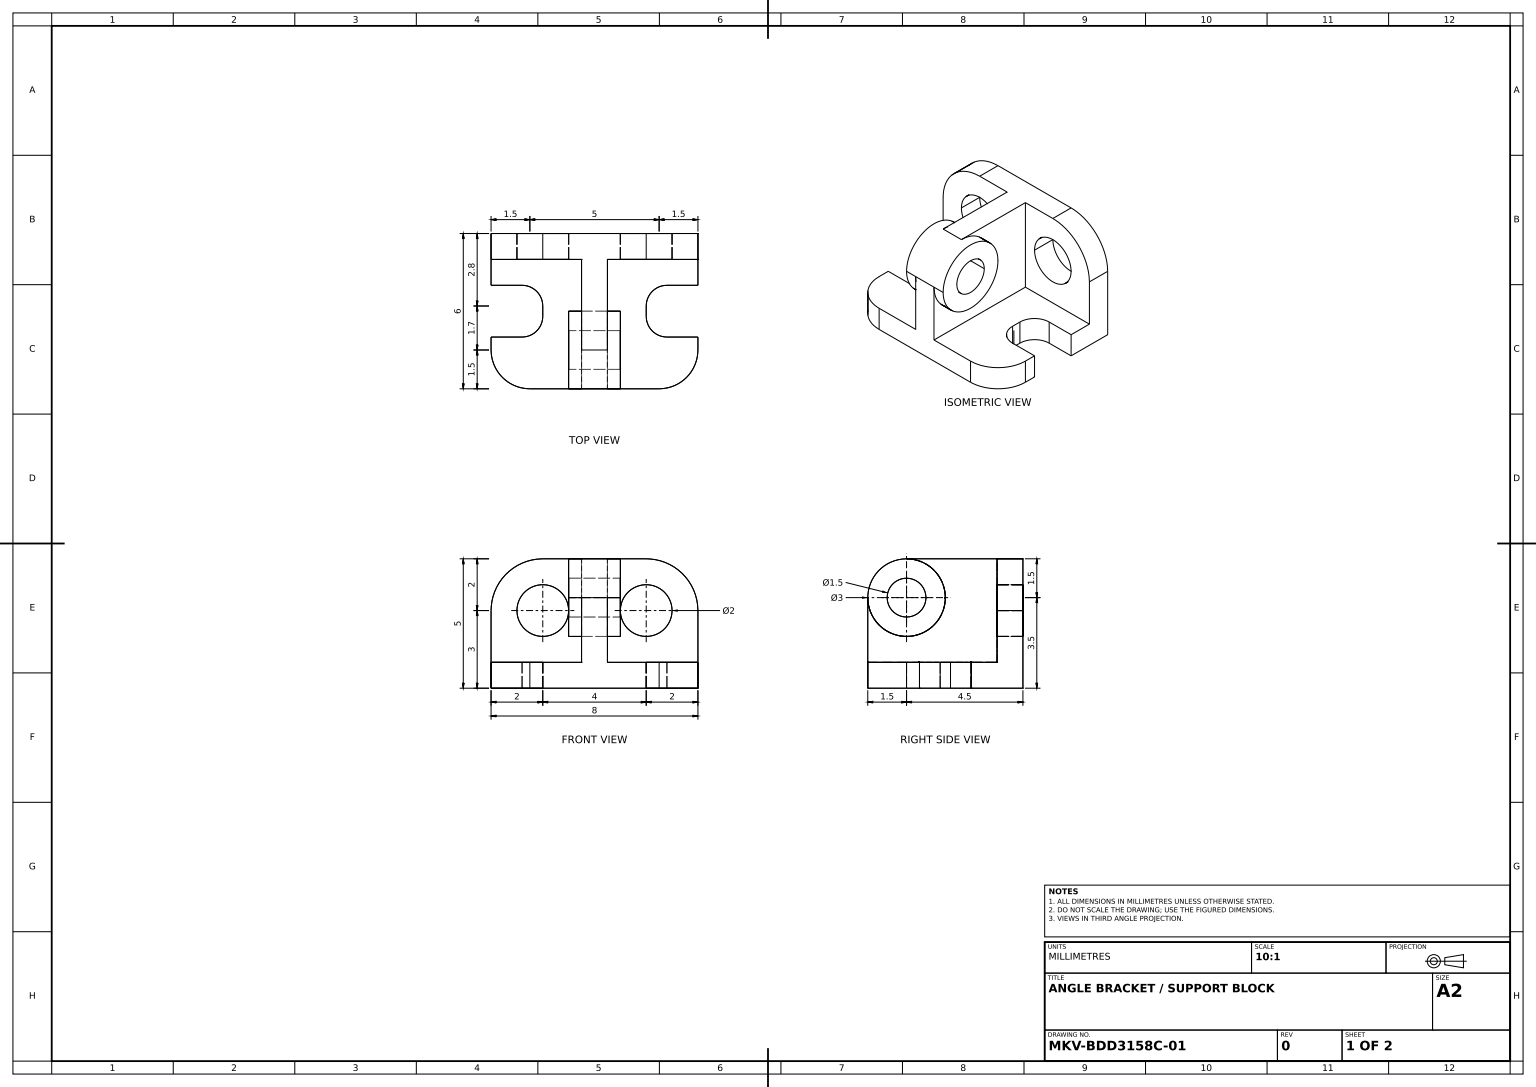
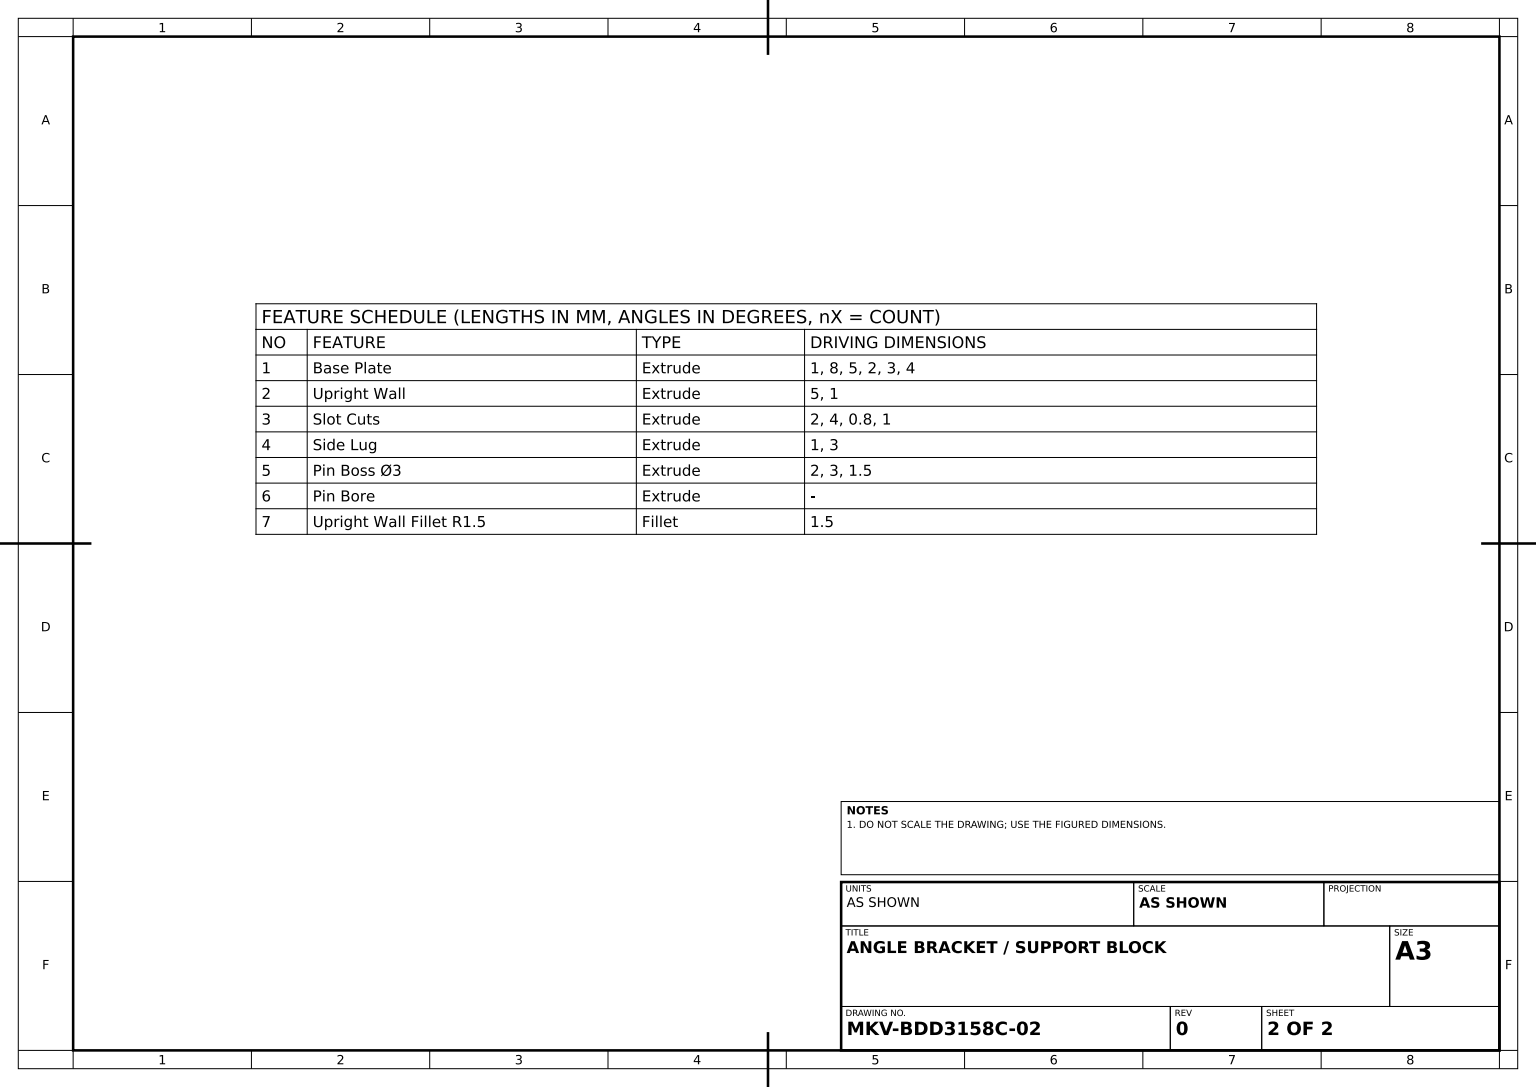
SolidWorks part; units mm, degrees
material "Plain Carbon Steel"
ref_plane "Front Plane" through (0, 0, 0) normal (0, 0, 1) x (1, 0, 0)
ref_plane "Top Plane" through (0, 0, 0) normal (0, 1, 0) x (1, 0, 0)
ref_plane "Right Plane" through (0, 0, 0) normal (1, 0, 0) x (0, 0, -1)
sketch "Base Plate Sketch" plane through (0, 0, 0) normal (0, 0, 1) x (1, 0, 0)
  line L1 (-2, 2.5) -> (2, 2.5)
  line L2 (-4, 0.5) -> (-4, -2.5)
  line L3 (-4, -2.5) -> (4, -2.5)
  line L4 (4, 0.5) -> (4, -2.5)
  line L5 (-4, 2.5) -> (4, -2.5) construction
  line L6 (-4, -2.5) -> (4, 2.5) construction
  arc A0 (-4, 0.5) -> (-2, 2.5) centre (-2, 0.5) cw
  arc A1 (4, 0.5) -> (2, 2.5) centre (2, 0.5) ccw
  circle A2 centre (-2, 0.5) radius 1
  circle A3 centre (2, 0.5) radius 1
  point P0 (0, 0)
  dimension "D3" = 2
  dimension "D4" = 2
  dimension "D5" = 2
  dimension "D6" = 2
  dimension "D8" = 3
  dimension "D1" = 8
  dimension "D2" = 5
  dimension "D7" = 3
  dimension "D9" = 4
  dimension "D10" = 2
extrude "Base Plate" add sketch "Base Plate Sketch" along normal blind 1
sketch "Upright Wall Sketch" plane through (0, 0, 1) normal (0, 0, 1) x (1, 0, 0)
  line L0 (4, -2.5) -> (4, 0.5) construction
  line L1 (-4, -2.5) -> (4, -2.5)
  line L2 (-4, -2.5) -> (-4, -1.5)
  line L3 (-4, -1.5) -> (4, -1.5)
  line L4 (4, -2.5) -> (4, -1.5)
  dimension "D1" = 1
extrude "Upright Wall" add sketch "Upright Wall Sketch" along normal blind 5
sketch "Slot Cuts Sketch" plane through (0, -1.5, 0) normal (0, 1, 0) x (1, 0, 0)
  line L1 (-4, -2) -> (-2.8, -2)
  line L2 (-4, -2) -> (-4, -4)
  line L3 (-4, -4) -> (-2.8, -4)
  line L4 (-2, -2.8) -> (-2, -3.2)
  line L5 (4, -2) -> (2.8, -2)
  line L6 (4, -2) -> (4, -4)
  line L7 (4, -4) -> (2.8, -4)
  line L8 (2, -2.8) -> (2, -3.2)
  line L9 (4, -6) -> (4, -1) construction
  line L10 (-4, -6) -> (-4, -1) construction
  line L11 (-4, -1) -> (-2, -1) construction
  line L12 (4, -1) -> (-4, -1) construction
  arc A0 (-2.8, -4) -> (-2, -3.2) centre (-2.8, -3.2) ccw
  arc A1 (-2, -2.8) -> (-2.8, -2) centre (-2.8, -2.8) ccw
  arc A2 (2.8, -4) -> (2, -3.2) centre (2.8, -3.2) cw
  arc A3 (2, -2.8) -> (2.8, -2) centre (2.8, -2.8) cw
  dimension "D10" = 0.8
  dimension "D1" = 2
  dimension "D2" = 2
  dimension "D3" = 1
  dimension "D4" = 1
  dimension "D5" = 4
  dimension "D6" = 2
  dimension "D7" = 2
  dimension "D8" = 0
  dimension "D9" = 0
extrude "Slot Cuts" cut sketch "Slot Cuts Sketch" against normal through all
sketch "Side Lug Sketch" plane through (0, 0, 0) normal (1, 0, 0) x (0, 0, -1)
  line L1 (-1, 2.5) -> (-4.5, 2.5)
  line L2 (-1, 2.5) -> (-1, -1.5)
  line L3 (-1, -1.5) -> (-6, -1.5)
  line L4 (-6, 1) -> (-6, -1.5)
  arc A1 (-4.5, 2.5) -> (-6, 1) centre (-4.5, 1) ccw
  dimension "D1" = 3
extrude "Side Lug" add sketch "Side Lug Sketch" along normal mid plane 1
sketch "Pin Boss Sketch" plane through (0, 0, 0) normal (1, 0, 0) x (0, 0, -1)
  line L0 (-6, 1) -> (-6, -1.5) construction
  line L1 (-1, 2.5) -> (-4.5, 2.5) construction
  circle A0 centre (-4.5, 1) radius 0.75
  circle A1 centre (-4.5, 1) radius 1.5
  dimension "D1" = 3
  dimension "D2" = 1.5
  dimension "D3" = 1.5
  dimension "D4" = 1.5
extrude "Pin Boss Ø3" add sketch "Pin Boss Sketch" along normal mid plane 2
sketch "Pin Bore Sketch" plane through (0.5, 0, 0) normal (1, 0, 0) x (0, 0, -1)
  circle A1 centre (-4.5, 1) radius 0.75
  circle A2 centre (-4.5, 1) radius 0.75
  dimension "D1" = 0
extrude "Pin Bore" cut sketch "Pin Bore Sketch" against normal through all contours A2
fillet "Upright Wall Fillet R1.5" radius 1.5 2 edges at (-4, -2, 6) (4, -2, 6)
